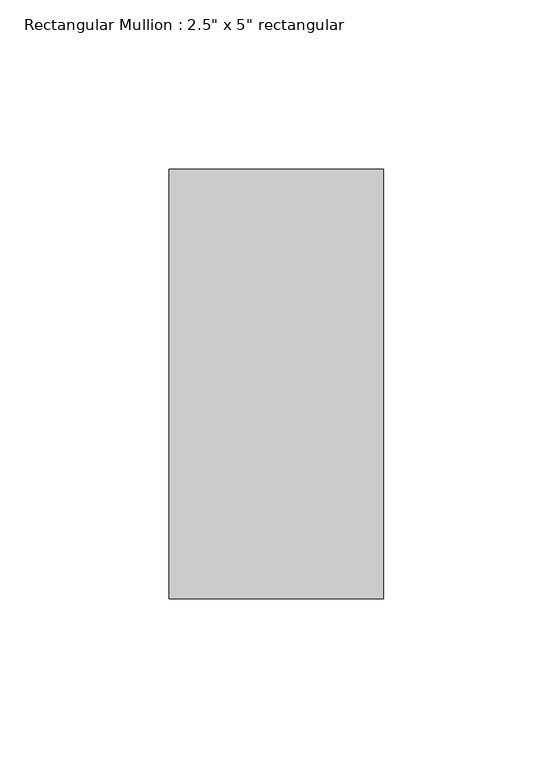
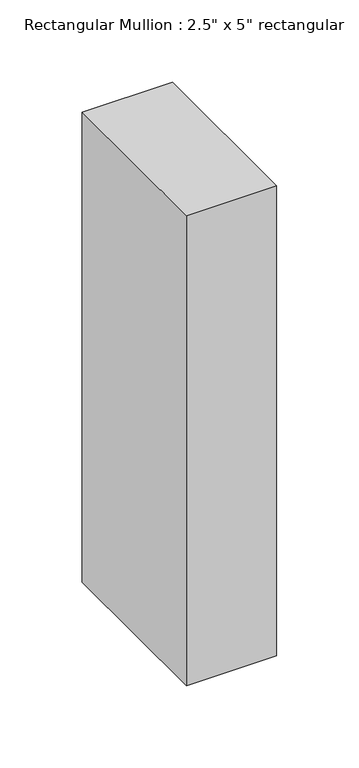
"""IFC4 building model written with IfcOpenShell, lengths in millimetres: member geometry."""

from ifc_helpers import new_model, si_unit, frame, origin, place, context, project, spatial, polyline, outline, extrude, source, transform, mapped, element, save


def member_585e2b51(model_context):
    return source(origin(), model_context, "Body", "SweptSolid", [
        extrude(outline(polyline([(31.75, 63.5), (31.75, -63.5), (-31.75, -63.5), (-31.75, 63.5), (31.75, 63.5)])), frame((0.0, 0.0, -349.25), z_axis=(0.0, 0.0, 1.0), x_axis=(1.0, 0.0, 0.0)), (0.0, 0.0, 1.0), 349.25),
    ])


if __name__ == "__main__":
    model = new_model("IFC4")
    model_context = context("Model", 3, world=origin())
    ifc_project = project(units=[si_unit("LENGTHUNIT", "METRE", prefix="MILLI")], contexts=[model_context])
    site = spatial("IfcSite", under=ifc_project)
    building = spatial("IfcBuilding", under=site)
    placement = place(None, origin())
    member_shape = member_585e2b51(model_context)
    element("IfcMember", 1, ObjectType="Rectangular Mullion : 2.5\" x 5\" rectangular", at=placement, inside=building, context=model_context, shape_type="MappedRepresentation", body=[
        mapped(member_shape, transform((0.0, 0.0, 0.0), x_axis=(1.0, 0.0, 0.0), y_axis=(0.0, 1.0, 0.0), z_axis=(0.0, 0.0, 1.0))),
    ])
    save(model, "model.ifc")

# Revit data of these elements
# Type "Rectangular Mullion : 2.5\" x 5\" rectangular"
#   built-in parameter 1007304 = 0.416667 (stored number, unit not read)
#   built-in parameter 1007301 = 0.104167 (stored number, unit not read)
#   built-in parameter 1007300 = 0.104167 (stored number, unit not read)
# Element 1 (IfcMember, "Rectangular Mullion : 2.5\" x 5\" rectangular")
#   Materials on its faces: "Aluminum"
# Materials
#   "Aluminum": class "Metal", colour RGB 247 247 247, transparency 0, Description = "Aluminum 6061", Cost = 0
